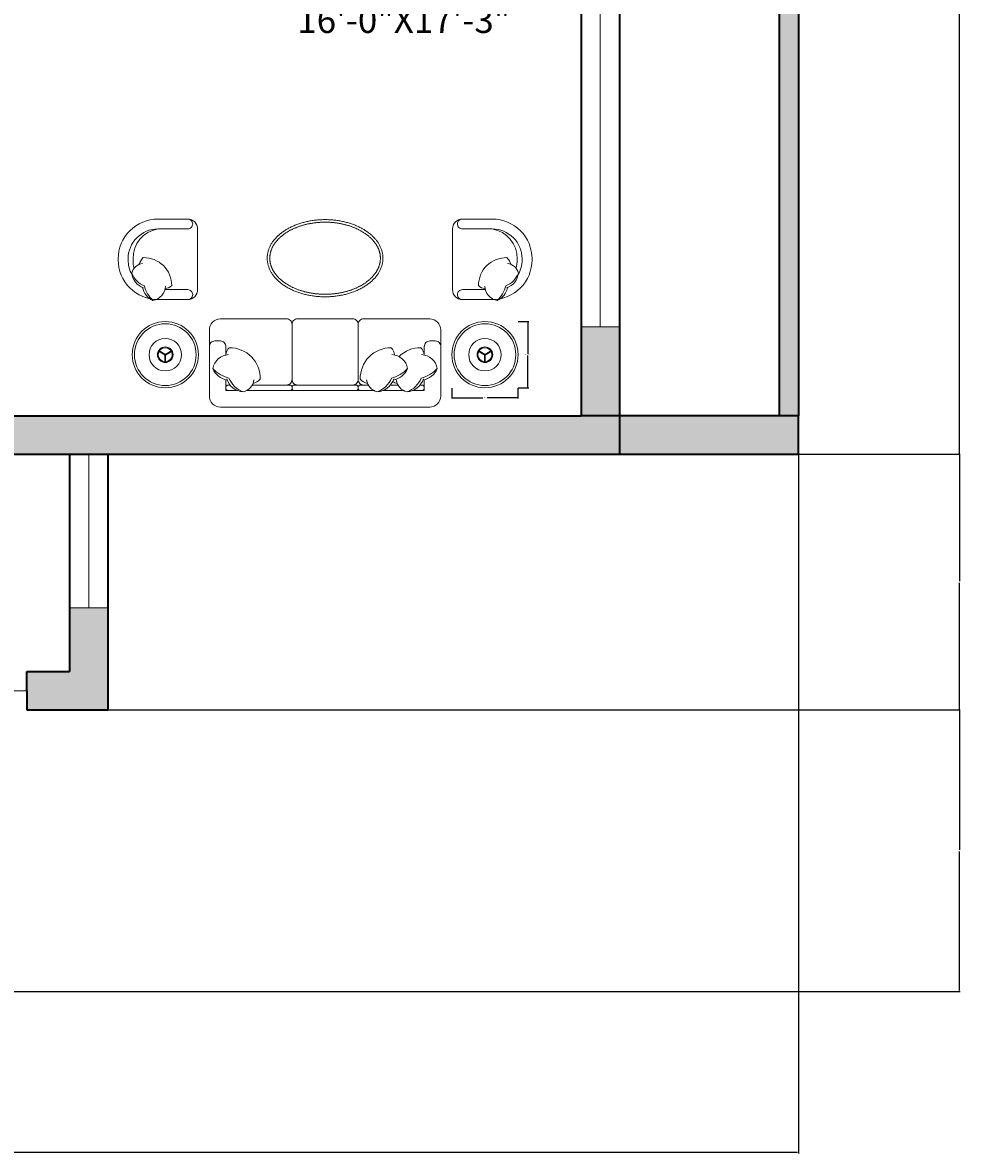
# Model space of a CAD drawing. Units: inches. Extents: x -36 to 442, y -676 to 151.
# Tile 2 of 8: x 222 to 442, y -676 to -411. Entities that reach past the tile are written whole.
import ezdxf

# ---------------------------------------------------------------- set-up
doc = ezdxf.new("R2010")
doc.units = ezdxf.units.IN
doc.header["$MEASUREMENT"] = 0
for name, color, linetype, lineweight in [('A-ANNO-DIMS', 2, 'Continuous', 18), ('A-AREA-IDEN', 7, 'Continuous', 18), ('A-DOOR', 4, 'Continuous', 18), ('A-FURN', 9, 'Continuous', 13), ('A-GLAZ', 4, 'Continuous', 13), ('A-WALL', 7, 'Continuous', 35), ('A-WALL-PATT', 8, 'Continuous', 13)]:
    doc.layers.add(name, color=color, linetype=linetype, lineweight=lineweight)
doc.styles.get("Standard").update_dxf_attribs({"font": 'arial.ttf'})
doc.dimstyles.get("Standard").update_dxf_attribs({"dimtxt": 0.18, "dimasz": 0.18, "dimexe": 0.18, "dimexo": 0.0625, "dimgap": 0.09, "dimtad": 0, "dimtih": 1, "dimtoh": 1, "dimdec": 0, "dimzin": 0, "dimdsep": 46, "dimlunit": 3, "dimtxsty": 'Standard', "dimcen": 0.09, "dimadec": 0, "dimazin": 0, "dimtfac": 1, "dimtdec": 0, "dimtofl": 0, "dimtmove": 0, "dimatfit": 3, "dimfxl": 1, "dimtolj": 1, "dimtzin": 0, "dimarcsym": 0})

# ---------------------------------------------------------------- blocks, each defined once
blk = doc.blocks.new('END-TABLE-ROUND')
at = {"ltscale": 0.03}
for p, q in [((7.72, 7.69), (6.14, 8.6)), ((7.8, 7.83), (6.22, 8.74)), ((7.72, 7.83), (9.3, 8.74)), ((7.8, 7.69), (9.38, 8.6)), ((7.68, 7.76), (7.68, 5.93)), ((7.84, 7.76), (7.84, 5.93))]:
    blk.add_line(p, q, dxfattribs=at)
for radius in [7.76, 3.81, 1.83, 1.64]:
    blk.add_circle((7.76, 7.76), radius, dxfattribs=at)
blk.add_circle((7.76, 7.76), 7.24)
blk = doc.blocks.new('GLAZING-UNIT-36IN')
for p, q in [((0, 36), (0, 0)), ((4.5, 36), (4.5, 0)), ((9, 0), (9, 36))]:
    blk.add_line(p, q)
blk = doc.blocks.new('GLAZING-UNIT-96IN')
for p, q in [((0, 0), (0, 96)), ((4.5, 96), (4.5, 0)), ((9, 96), (9, 0))]:
    blk.add_line(p, q)
blk = doc.blocks.new('*D41')
at = {"layer": 'A-ANNO-DIMS', "color": 0, "lineweight": -2, "transparency": 16777216}
for p, q in [((338.51, -480.93), (340.96, -480.93)), ((340.78, -481.11), (340.78, -488.51)), ((340.78, -496.27), (340.78, -488.87)), ((338.51, -496.45), (340.96, -496.45))]:
    blk.add_line(p, q, dxfattribs=at)
at = {"layer": 'A-ANNO-DIMS', "color": 0, "transparency": 16777216}
for points in [[(340.75, -481.11), (340.81, -481.11), (340.78, -480.93)], [(340.75, -496.27), (340.81, -496.27), (340.78, -496.45)]]:
    blk.add_solid(points, dxfattribs=at)
at = {"layer": 'Defpoints', "color": 0, "transparency": 16777216}
for p in [(338.45, -480.93), (340.78, -480.93), (338.45, -496.45)]:
    blk.add_point(p, dxfattribs=at)
at = {"layer": 'A-ANNO-DIMS', "color": 0, "transparency": 16777216, "insert": (340.78, -488.69), "char_height": 0.18, "attachment_point": 5}
blk.add_mtext('\\A1;TABLE 16 TYP.', dxfattribs=at)
blk = doc.blocks.new('*D42')
at = {"layer": 'A-ANNO-DIMS', "color": 0, "lineweight": -2, "transparency": 16777216}
for p, q in [((322.94, -496.51), (322.94, -498.96)), ((338.45, -496.51), (338.45, -498.96)), ((323.12, -498.78), (330.17, -498.78)), ((338.27, -498.78), (331.21, -498.78))]:
    blk.add_line(p, q, dxfattribs=at)
at = {"layer": 'A-ANNO-DIMS', "color": 0, "transparency": 16777216}
for points in [[(323.12, -498.75), (323.12, -498.81), (322.94, -498.78)], [(338.27, -498.75), (338.27, -498.81), (338.45, -498.78)]]:
    blk.add_solid(points, dxfattribs=at)
at = {"layer": 'Defpoints', "color": 0, "transparency": 16777216}
for p in [(322.94, -496.45), (338.45, -496.45), (338.45, -498.78)]:
    blk.add_point(p, dxfattribs=at)
at = {"layer": 'A-ANNO-DIMS', "color": 0, "transparency": 16777216, "insert": (330.69, -498.78), "char_height": 0.18, "attachment_point": 5}
blk.add_mtext('\\A1;16 TYP.', dxfattribs=at)
blk = doc.blocks.new('*D49')
at = {"layer": 'A-ANNO-DIMS', "color": 0, "lineweight": -2, "transparency": 16777216}
for p, q in [((2.24, -363.56), (2.24, -675.98)), ((404.24, -512.06), (404.24, -675.98)), ((2.42, -675.8), (202.94, -675.8)), ((404.06, -675.8), (203.53, -675.8))]:
    blk.add_line(p, q, dxfattribs=at)
at = {"layer": 'A-ANNO-DIMS', "color": 0, "transparency": 16777216}
for points in [[(2.42, -675.77), (2.42, -675.83), (2.24, -675.8)], [(404.06, -675.77), (404.06, -675.83), (404.24, -675.8)]]:
    blk.add_solid(points, dxfattribs=at)
at = {"layer": 'Defpoints', "color": 0, "transparency": 16777216}
for p in [(2.24, -363.5), (404.24, -512), (404.24, -675.8)]:
    blk.add_point(p, dxfattribs=at)
at = {"layer": 'A-ANNO-DIMS', "color": 0, "transparency": 16777216, "insert": (203.24, -675.8), "char_height": 0.18, "attachment_point": 5}
blk.add_mtext('\\A1;402', dxfattribs=at)
blk = doc.blocks.new('*D59')
at = {"layer": 'A-ANNO-DIMS', "color": 0, "lineweight": -2, "transparency": 16777216}
for p, q in [((404.3, -287), (442.22, -287)), ((442.04, -287.18), (442.04, -399.32)), ((442.04, -511.82), (442.04, -399.68)), ((404.3, -512), (442.22, -512))]:
    blk.add_line(p, q, dxfattribs=at)
at = {"layer": 'A-ANNO-DIMS', "color": 0, "transparency": 16777216}
for points in [[(442.01, -287.18), (442.07, -287.18), (442.04, -287)], [(442.01, -511.82), (442.07, -511.82), (442.04, -512)]]:
    blk.add_solid(points, dxfattribs=at)
at = {"layer": 'Defpoints', "color": 0, "transparency": 16777216}
for p in [(404.24, -287), (404.24, -512), (442.04, -512)]:
    blk.add_point(p, dxfattribs=at)
at = {"layer": 'A-ANNO-DIMS', "color": 0, "transparency": 16777216, "insert": (442.04, -399.5), "char_height": 0.18, "attachment_point": 5}
blk.add_mtext('\\A1;225', dxfattribs=at)
blk = doc.blocks.new('*D60')
at = {"layer": 'A-ANNO-DIMS', "color": 0, "lineweight": -2, "transparency": 16777216}
for p, q in [((404.3, -512), (442.22, -512)), ((442.04, -512.18), (442.04, -541.82)), ((442.04, -571.82), (442.04, -542.18)), ((242.3, -572), (442.22, -572))]:
    blk.add_line(p, q, dxfattribs=at)
at = {"layer": 'A-ANNO-DIMS', "color": 0, "transparency": 16777216}
for points in [[(442.01, -512.18), (442.07, -512.18), (442.04, -512)], [(442.01, -571.82), (442.07, -571.82), (442.04, -572)]]:
    blk.add_solid(points, dxfattribs=at)
at = {"layer": 'Defpoints', "color": 0, "transparency": 16777216}
for p in [(404.24, -512), (442.04, -512), (242.24, -572)]:
    blk.add_point(p, dxfattribs=at)
at = {"layer": 'A-ANNO-DIMS', "color": 0, "transparency": 16777216, "insert": (442.04, -542), "char_height": 0.18, "attachment_point": 5}
blk.add_mtext('\\A1;60', dxfattribs=at)
blk = doc.blocks.new('*D61')
at = {"layer": 'A-ANNO-DIMS', "color": 0, "lineweight": -2, "transparency": 16777216}
for p, q in [((242.3, -572), (442.22, -572)), ((442.04, -572.18), (442.04, -604.82)), ((442.04, -637.82), (442.04, -605.18)), ((72.8, -638), (442.22, -638))]:
    blk.add_line(p, q, dxfattribs=at)
at = {"layer": 'A-ANNO-DIMS', "color": 0, "transparency": 16777216}
for points in [[(442.01, -572.18), (442.07, -572.18), (442.04, -572)], [(442.01, -637.82), (442.07, -637.82), (442.04, -638)]]:
    blk.add_solid(points, dxfattribs=at)
at = {"layer": 'Defpoints', "color": 0, "transparency": 16777216}
for p in [(242.24, -572), (442.04, -572), (72.74, -638)]:
    blk.add_point(p, dxfattribs=at)
at = {"layer": 'A-ANNO-DIMS', "color": 0, "transparency": 16777216, "insert": (442.04, -605), "char_height": 0.18, "attachment_point": 5}
blk.add_mtext('\\A1;66', dxfattribs=at)

msp = doc.modelspace()

# ---------------------------------------------------------------- hatches: boundary and pattern name
at = {"layer": 'A-WALL-PATT'}
h = msp.add_hatch(color=256, dxfattribs=at)
h.dxf.hatch_style = 1
h.paths.add_polyline_path([(288, 113.503), (193.5, 113.503), (97.5, 113.503), (97.5, 104.864), (106.5, 104.864), (106.5, 104.503), (193.5, 104.503), (193.5, 5.503), (193.5, 1.003), (213.735, 1.003), (213.735, -135.497), (218.235, -135.497), (218.235, 1.003), (251, 1.003), (251, 3.253), (251, 5.503), (198, 5.503), (198, 104.503), (279, 104.503), (279, 104.209), (288, 104.209)])
h.paths.add_polyline_path([(378.735, 81.646), (362.235, 81.646), (288, 81.646), (288, 80.209), (279, 80.209), (279, 5.503), (279, 1.003), (353.235, 1.003), (353.235, 0.242), (362.235, 0.242), (362.235, 5.503), (288, 5.503), (288, 77.146), (362.235, 77.146), (374.235, 77.146), (374.235, 5.503), (362.235, 5.503), (362.235, 1.003), (374.235, 1.003), (378.735, 1.003), (378.735, 5.503), (378.735, 77.146)])
h.paths.add_polyline_path([(362.235, -35.758), (353.235, -35.758), (353.235, -196.997), (218.235, -196.997), (213.735, -196.997), (213.735, -205.997), (218.235, -205.997), (378.735, -205.997), (378.735, -205.779), (387.735, -205.779), (387.735, -202.472), (387.735, -196.997), (378.735, -196.997), (362.235, -196.997)])
h.paths.add_polyline_path([(218.235, -175.497), (215.985, -175.497), (213.735, -175.497), (213.735, -196.997), (218.235, -196.997)], flags=17)
h.paths.add_polyline_path([(158.235, -201.497), (98.235, -201.497), (98.235, -205.997), (158.235, -205.997)])
h.paths.add_polyline_path([(173.735, -130.997), (27.735, -130.997), (27.735, -35.267), (18.735, -35.267), (18.735, -138.68), (27.735, -138.68), (27.735, -135.497), (93.735, -135.497), (93.735, -201.497), (98.235, -201.497), (98.235, -135.497), (158.235, -135.497), (158.235, -173.497), (160.739, -173.497), (162.735, -173.497), (162.735, -135.497), (173.735, -135.497), (173.735, -133.017)])
h.paths.add_polyline_path([(98.235, -201.497), (93.735, -201.497), (93.735, -205.997), (98.235, -205.997)])
h.paths.add_polyline_path([(162.735, -201.497), (158.235, -201.497), (158.235, -205.997), (162.735, -205.997)])
h.paths.add_polyline_path([(63.735, -205.997), (63.735, -201.497), (27.735, -201.497), (27.735, -162.68), (18.735, -162.68), (18.735, -210.497), (63.735, -210.497)])
h.paths.add_polyline_path([(65.735, -203.604), (65.735, -201.497), (63.735, -201.497), (63.735, -205.997), (65.735, -205.997)])
h.paths.add_polyline_path([(165.5, 5.503), (106.5, 5.503), (106.5, 80.864), (97.5, 80.864), (97.5, 81.646), (6.735, 81.646), (2.235, 81.646), (2.235, 77.146), (2.235, 5.503), (2.235, 1.003), (6.735, 1.003), (18.735, 1.003), (18.735, 5.503), (6.735, 5.503), (6.735, 77.146), (97.5, 77.146), (97.5, 5.503), (18.735, 5.503), (18.735, 0.733), (27.735, 0.733), (27.735, 1.003), (165.5, 1.003), (165.5, 3.253)])
h.paths.add_polyline_path([(18.735, -201.497), (6.735, -201.497), (2.235, -201.497), (2.235, -210.497), (2.235, -354.497), (2.235, -363.497), (6.735, -363.497), (18.735, -363.497), (18.735, -358.997), (18.735, -354.497), (6.735, -354.497), (6.735, -210.497), (18.735, -210.497)])
h.paths.add_polyline_path([(63.735, -210.497), (54.735, -210.497), (54.735, -240.747), (63.735, -240.747)])
h.paths.add_polyline_path([(63.735, -336.747), (54.735, -336.747), (54.735, -354.497), (18.735, -354.497), (18.735, -358.997), (18.735, -363.497), (104.735, -363.497), (104.735, -361.247), (104.735, -358.997), (63.735, -358.997)])
h.paths.add_polyline_path([(27.735, -448.151), (18.735, -448.151), (18.735, -637.997), (72.735, -637.997), (72.735, -571.997), (183.235, -571.997), (183.235, -562.997), (57.197, -562.997), (51.735, -562.997), (51.735, -567.497), (57.197, -567.497), (63.735, -567.497), (63.735, -571.997), (63.735, -628.997), (27.735, -628.997), (27.735, -475.997), (27.735, -471.497)])
h.paths.add_polyline_path([(27.735, -363.497), (18.735, -363.497), (18.735, -412.151), (27.735, -412.151)])
h.paths.add_polyline_path([(161.235, -358.997), (132.735, -358.997), (132.735, -363.497), (156.735, -363.497), (156.735, -471.497), (51.735, -471.497), (51.735, -475.997), (63.735, -475.997), (63.735, -534.997), (65.985, -534.997), (68.235, -534.997), (68.235, -475.997), (161.235, -475.997)])
h.paths.add_polyline_path([(161.235, -511.997), (173.235, -511.997), (173.235, -502.997), (161.235, -502.997), (161.235, -475.997), (152.235, -475.997), (152.235, -534.997), (156.735, -534.997), (161.235, -534.997)], flags=17)
h.paths.add_polyline_path([(362.235, -502.997), (353.235, -502.997), (213.235, -502.997), (213.235, -507.497), (213.235, -511.997), (362.235, -511.997)])
h.paths.add_polyline_path([(242.235, -548.019), (233.235, -548.019), (233.235, -562.997), (223.235, -562.997), (223.235, -567.497), (223.235, -571.997), (242.235, -571.997)])
h.paths.add_polyline_path([(404.235, -502.997), (399.735, -502.997), (362.235, -502.997), (362.235, -511.997), (399.735, -511.997), (404.235, -511.997)])
h.paths.add_polyline_path([(362.235, -482.123), (353.235, -482.123), (353.235, -502.997), (362.235, -502.997)])
h.paths.add_polyline_path([(404.235, -295.997), (404.235, -286.997), (387.735, -286.997), (387.735, -295.997), (399.735, -295.997), (399.735, -502.997), (404.235, -502.997)])
h.paths.add_polyline_path([(362.235, -355.863), (353.235, -355.863), (353.235, -386.123), (362.235, -386.123)])
h.paths.add_polyline_path([(387.735, -286.997), (378.735, -286.997), (213.735, -286.997), (213.735, -295.997), (353.235, -295.997), (353.235, -295.863), (362.235, -295.863), (362.235, -295.997), (378.735, -295.997), (387.735, -295.997)])
h.paths.add_polyline_path([(387.735, -241.779), (378.735, -241.779), (378.735, -286.997), (387.735, -286.997)])
h.paths.add_polyline_path([(387.735, -175.497), (362.235, -175.497), (362.235, -184.497), (387.735, -184.497)], flags=17)
h.paths.add_polyline_path([(387.735, -184.497), (383.235, -184.497), (383.235, -192.497), (378.735, -192.497), (366.735, -192.497), (366.735, -184.497), (362.235, -184.497), (362.235, -196.997), (378.735, -196.997), (387.735, -196.997)], flags=17)
h.paths.add_polyline_path([(240.604, 40.967), (282.575, 40.967), (282.575, 63.356), (240.604, 63.356)], flags=25)

# ---------------------------------------------------------------- linework, layer by layer
at = {"layer": 'A-DOOR'}
msp.add_line((220.235, -567.497), (223.235, -567.497), dxfattribs=at)
at = {"layer": 'A-FURN', "ltscale": 0.03}
for points in [[(263.302, -466.323), (263.302, -459.212, 0.4142136), (260.97, -456.88), (253.975, -456.88, 0.4142136), (244.649, -466.207), (244.649, -466.323), (244.649, -466.44, 0.4142136), (253.975, -475.766), (260.97, -475.766, 0.4142136), (263.302, -473.435), (263.302, -466.323)], [(323.093, -466.323), (323.093, -459.212, -0.4142136), (325.425, -456.88), (332.42, -456.88, -0.4142136), (341.746, -466.207), (341.746, -466.323), (341.746, -466.44, -0.4142136), (332.42, -475.766), (325.425, -475.766, -0.4142136), (323.093, -473.435), (323.093, -466.323)]]:
    msp.add_lwpolyline(points, format="xyb", dxfattribs=at)
at = {"layer": 'A-FURN'}
for points in [[(253.975, -459.212), (260.97, -459.212, 0.4142136), (262.136, -458.046), (262.136, -458.046, 0.4142136), (260.97, -456.88)], [(332.42, -459.212), (325.425, -459.212, -0.4142136), (324.259, -458.046), (324.259, -458.046, -0.4142136), (325.425, -456.88)], [(253.975, -459.212, 0.4142136), (246.98, -466.207), (246.98, -466.323)], [(253.975, -459.212, 0.3727189), (248.146, -466.207), (248.146, -466.323)], [(332.42, -459.212, -0.3727189), (338.249, -466.207), (338.249, -466.323)], [(332.42, -459.212, -0.4142136), (339.414, -466.207), (339.414, -466.323)], [(247.903, -469.912, -0.1305915), (246.98, -466.44), (246.98, -466.323)], [(248.397, -468.427, -0.0723842), (248.146, -466.44), (248.146, -466.323)], [(255.666, -473.204, 0.1655406), (257.206, -472.483, 0.4259892), (250.528, -465.935, 0.1215233), (249.607, -467.49, -7.1154643)], [(330.729, -473.204, -0.1655406), (329.189, -472.483, -0.4259892), (335.867, -465.935, -0.1215233), (336.788, -467.49, 7.1154643)], [(337.997, -468.427, 0.0723842), (338.249, -466.44), (338.249, -466.323)], [(338.492, -469.912, 0.1305915), (339.414, -466.44), (339.414, -466.323)], [(250.635, -473.02, -0.3066635), (247.856, -469.543, -0.30633), (250.394, -467.272, 0.8728472)], [(335.76, -473.02, 0.3066635), (338.538, -469.543, 0.30633), (336.001, -467.272, -0.8728472)], [(252.798, -475.957, -0.1477299), (250.795, -472.55, -0.2133428), (247.856, -469.543, -0.1786618)], [(333.596, -475.957, 0.1477299), (335.6, -472.55, 0.2133428), (338.538, -469.543, 0.1786618)], [(255.737, -472.616, -0.3567724), (252.798, -475.957, -0.2495421), (250.377, -472.93, 9.6168803)], [(255.61, -473.435), (260.97, -473.435, -0.4142136), (262.136, -474.601), (262.136, -474.601, -0.4142136), (260.97, -475.766)], [(330.785, -473.435), (325.425, -473.435, 0.4142136), (324.259, -474.601), (324.259, -474.601, 0.4142136), (325.425, -475.766)], [(330.658, -472.616, 0.3567724), (333.596, -475.957, 0.2495421), (336.018, -472.93, -9.6168803)], [(284.146, -495.803, 0.4142136), (285.439, -494.51), (285.439, -481.581, 0.4142136)], [(302.248, -495.803, -0.4142136), (300.955, -494.51), (300.955, -481.581, -0.4142136)], [(266.044, -486.753, -0.4142136), (267.337, -485.46), (268.63, -485.46, -0.4142136), (269.923, -486.753), (269.923, -488.756)], [(269.921, -488.756, -0.1655406), (270.721, -487.048, -0.4259892), (277.982, -494.455, -0.1215233), (276.258, -495.476, 7.1154643)], [(309.509, -488.756, 0.1655406), (308.709, -487.048, 0.4259892), (301.447, -494.455, 0.1215233), (303.171, -495.476, -7.1154643)], [(316.474, -488.756, 0.1655406), (315.674, -487.048, 0.2002311), (310.541, -489.129, 0.1215233)], [(316.471, -488.756), (316.471, -486.753, -0.4142136), (317.764, -485.46), (319.057, -485.46, -0.4142136), (320.35, -486.753)], [(270.572, -488.678, 0.3567724), (266.867, -491.937, 0.2495421), (270.224, -494.623, -9.6168803)], [(308.857, -488.678, -0.3567724), (312.562, -491.937, -0.2495421), (309.205, -494.623, 9.6168803)], [(315.822, -488.678, -0.3567724), (319.527, -491.937, -0.2495421), (316.17, -494.623, 9.6168803)], [(266.867, -491.937, 0.1477299), (270.646, -494.159, 0.2133428), (273.981, -497.418, 0.1786618)], [(312.562, -491.937, -0.1477299), (308.783, -494.159, -0.2133428), (305.449, -497.418, -0.1786618)], [(319.527, -491.937, -0.1477299), (315.748, -494.159, -0.2133428), (312.414, -497.418, -0.1786618)], [(270.91, -495.803), (270.441, -495.803, 0.4142136), (269.923, -496.321), (269.923, -496.579, 0.4142136), (270.441, -497.096)], [(270.124, -494.336, 0.3066635), (273.981, -497.418, 0.30633), (276.5, -494.603, -0.8728472)], [(274.795, -497.096), (284.922, -497.096, 0.4142136), (285.439, -496.579), (285.439, -496.321, 0.4142136), (284.922, -495.803), (276.097, -495.803, 0.4142136)], [(286.732, -495.803, -0.4142136), (285.439, -494.51)], [(299.662, -495.803, 0.4142136), (300.955, -494.51)], [(304.635, -497.096), (301.473, -497.096, -0.4142136), (300.955, -496.579), (300.955, -496.321, -0.4142136), (301.473, -495.803), (303.333, -495.803, -0.4142136)], [(309.305, -494.336, -0.3066635), (305.449, -497.418, -0.30633), (302.929, -494.603, 0.8728472)], [(308.519, -495.803), (310.298, -495.803, -0.4142136)], [(309.052, -494.971, 0.0718654), (310.136, -495.476, -7.1154643)], [(316.27, -494.336, -0.3066635), (312.414, -497.418, -0.30633), (309.894, -494.603, 0.8728472)], [(313.751, -497.096), (316.471, -497.096), (316.471, -494.555, -0.4142136)], [(315.485, -495.803), (315.954, -495.803, -0.4142136), (316.471, -496.321), (316.471, -496.579, -0.4142136), (315.954, -497.096)], [(270.441, -497.096), (272.644, -497.096, 0.4142136)], [(311.6, -497.096), (306.786, -497.096, -0.4142136)], [(315.954, -497.096), (313.751, -497.096, -0.4142136)]]:
    msp.add_lwpolyline(points, format="xyb", dxfattribs=at)
at = {"layer": 'A-FURN', "ltscale": 0.03}
msp.add_lwpolyline([(266.044, -482.874, -0.4142136), (268.63, -480.288), (284.146, -480.288, -0.4142136), (285.439, -481.581, -0.4142136), (286.732, -480.288), (299.662, -480.288, -0.4142136), (300.955, -481.581, -0.4142136), (302.248, -480.288), (317.764, -480.288, -0.4142136), (320.35, -482.874), (320.35, -498.389, -0.4142136), (317.764, -500.975), (268.63, -500.975, -0.4142136), (266.044, -498.389)], format="xyb", close=True, dxfattribs=at)
at = {"layer": 'A-FURN'}
for points in [[(269.923, -494.555), (269.923, -497.096), (272.644, -497.096)], [(274.795, -497.096), (304.635, -497.096)], [(306.786, -497.096), (311.6, -497.096)]]:
    msp.add_lwpolyline(points, dxfattribs=at)
msp.add_lwpolyline([(300.438, -497.096), (285.957, -497.096, -0.4142136), (285.439, -496.579), (285.439, -496.321, -0.4142136), (285.957, -495.803), (300.438, -495.803, -0.4142136), (300.955, -496.321), (300.955, -496.579, -0.4142136)], format="xyb", close=True, dxfattribs=at)
at = {"layer": 'A-FURN', "ltscale": 0.03}
msp.add_polyline3d([(279.621, -466.065, 0), (279.623, -466.236, 0), (279.631, -466.407, 0), (279.643, -466.578, 0), (279.66, -466.749, 0), (279.682, -466.92, 0), (279.708, -467.09, 0), (279.74, -467.26, 0), (279.776, -467.43, 0), (279.817, -467.599, 0), (279.863, -467.767, 0), (279.914, -467.935, 0), (279.97, -468.103, 0), (280.03, -468.269, 0), (280.095, -468.435, 0), (280.164, -468.6, 0), (280.239, -468.764, 0), (280.318, -468.927, 0), (280.401, -469.089, 0), (280.489, -469.249, 0), (280.582, -469.409, 0), (280.679, -469.568, 0), (280.781, -469.725, 0), (280.887, -469.881, 0), (280.997, -470.036, 0), (281.112, -470.189, 0), (281.232, -470.341, 0), (281.355, -470.491, 0), (281.483, -470.639, 0), (281.615, -470.786, 0), (281.751, -470.932, 0), (281.891, -471.075, 0), (282.035, -471.217, 0), (282.184, -471.357, 0), (282.336, -471.495, 0), (282.492, -471.631, 0), (282.652, -471.765, 0), (282.816, -471.897, 0), (282.983, -472.027, 0), (283.154, -472.155, 0), (283.329, -472.28, 0), (283.507, -472.404, 0), (283.689, -472.525, 0), (283.874, -472.644, 0), (284.062, -472.76, 0), (284.254, -472.874, 0), (284.449, -472.986, 0), (284.647, -473.095, 0), (284.848, -473.202, 0), (285.052, -473.306, 0), (285.259, -473.407, 0), (285.469, -473.506, 0), (285.681, -473.602, 0), (285.897, -473.696, 0), (286.115, -473.786, 0), (286.335, -473.874, 0), (286.558, -473.959, 0), (286.783, -474.042, 0), (287.011, -474.121, 0), (287.241, -474.198, 0), (287.473, -474.272, 0), (287.707, -474.342, 0), (287.943, -474.41, 0), (288.18, -474.475, 0), (288.42, -474.537, 0), (288.661, -474.595, 0), (288.904, -474.651, 0), (289.149, -474.704, 0), (289.395, -474.753, 0), (289.642, -474.8, 0), (289.891, -474.843, 0), (290.141, -474.883, 0), (290.391, -474.92, 0), (290.643, -474.954, 0), (290.896, -474.985, 0), (291.15, -475.012, 0), (291.404, -475.036, 0), (291.659, -475.057, 0), (291.915, -475.075, 0), (292.171, -475.09, 0), (292.427, -475.101, 0), (292.684, -475.109, 0), (292.94, -475.114, 0), (293.197, -475.116, 0), (293.454, -475.114, 0), (293.711, -475.109, 0), (293.968, -475.101, 0), (294.224, -475.09, 0), (294.48, -475.075, 0), (294.736, -475.057, 0), (294.991, -475.036, 0), (295.245, -475.012, 0), (295.499, -474.985, 0), (295.751, -474.954, 0), (296.003, -474.92, 0), (296.254, -474.883, 0), (296.504, -474.843, 0), (296.753, -474.8, 0), (297, -474.753, 0), (297.246, -474.704, 0), (297.49, -474.651, 0), (297.733, -474.595, 0), (297.975, -474.537, 0), (298.214, -474.475, 0), (298.452, -474.41, 0), (298.688, -474.342, 0), (298.922, -474.272, 0), (299.154, -474.198, 0), (299.384, -474.121, 0), (299.611, -474.042, 0), (299.837, -473.959, 0), (300.06, -473.874, 0), (300.28, -473.786, 0), (300.498, -473.696, 0), (300.713, -473.602, 0), (300.926, -473.506, 0), (301.136, -473.407, 0), (301.343, -473.306, 0), (301.547, -473.202, 0), (301.748, -473.095, 0), (301.946, -472.986, 0), (302.141, -472.874, 0), (302.333, -472.76, 0), (302.521, -472.644, 0), (302.706, -472.525, 0), (302.888, -472.404, 0), (303.066, -472.28, 0), (303.241, -472.155, 0), (303.412, -472.027, 0), (303.579, -471.897, 0), (303.743, -471.765, 0), (303.903, -471.631, 0), (304.059, -471.495, 0), (304.211, -471.357, 0), (304.359, -471.217, 0), (304.504, -471.075, 0), (304.644, -470.932, 0), (304.78, -470.786, 0), (304.912, -470.639, 0), (305.04, -470.491, 0), (305.163, -470.341, 0), (305.282, -470.189, 0), (305.397, -470.036, 0), (305.508, -469.881, 0), (305.614, -469.725, 0), (305.716, -469.568, 0), (305.813, -469.409, 0), (305.906, -469.249, 0), (305.994, -469.089, 0), (306.077, -468.927, 0), (306.156, -468.764, 0), (306.23, -468.6, 0), (306.3, -468.435, 0), (306.365, -468.269, 0), (306.425, -468.103, 0), (306.481, -467.935, 0), (306.531, -467.767, 0), (306.577, -467.599, 0), (306.618, -467.43, 0), (306.655, -467.26, 0), (306.686, -467.09, 0), (306.713, -466.92, 0), (306.735, -466.749, 0), (306.752, -466.578, 0), (306.764, -466.407, 0), (306.771, -466.236, 0), (306.774, -466.065, 0), (306.771, -465.893, 0), (306.764, -465.722, 0), (306.752, -465.551, 0), (306.735, -465.38, 0), (306.713, -465.209, 0), (306.686, -465.039, 0), (306.655, -464.869, 0), (306.618, -464.7, 0), (306.577, -464.53, 0), (306.531, -464.362, 0), (306.481, -464.194, 0), (306.425, -464.027, 0), (306.365, -463.86, 0), (306.3, -463.695, 0), (306.23, -463.53, 0), (306.156, -463.366, 0), (306.077, -463.203, 0), (305.994, -463.041, 0), (305.906, -462.88, 0), (305.813, -462.72, 0), (305.716, -462.561, 0), (305.614, -462.404, 0), (305.508, -462.248, 0), (305.397, -462.094, 0), (305.282, -461.94, 0), (305.163, -461.789, 0), (305.04, -461.638, 0), (304.912, -461.49, 0), (304.78, -461.343, 0), (304.644, -461.198, 0), (304.504, -461.054, 0), (304.359, -460.912, 0), (304.211, -460.772, 0), (304.059, -460.634, 0), (303.903, -460.498, 0), (303.743, -460.364, 0), (303.579, -460.232, 0), (303.412, -460.102, 0), (303.241, -459.974, 0), (303.066, -459.849, 0), (302.888, -459.725, 0), (302.706, -459.604, 0), (302.521, -459.486, 0), (302.333, -459.369, 0), (302.141, -459.255, 0), (301.946, -459.143, 0), (301.748, -459.034, 0), (301.547, -458.928, 0), (301.343, -458.824, 0), (301.136, -458.722, 0), (300.926, -458.623, 0), (300.713, -458.527, 0), (300.498, -458.434, 0), (300.28, -458.343, 0), (300.06, -458.255, 0), (299.837, -458.17, 0), (299.611, -458.087, 0), (299.384, -458.008, 0), (299.154, -457.931, 0), (298.922, -457.858, 0), (298.688, -457.787, 0), (298.452, -457.719, 0), (298.214, -457.654, 0), (297.975, -457.593, 0), (297.733, -457.534, 0), (297.49, -457.478, 0), (297.246, -457.425, 0), (297, -457.376, 0), (296.753, -457.33, 0), (296.504, -457.286, 0), (296.254, -457.246, 0), (296.003, -457.209, 0), (295.751, -457.175, 0), (295.499, -457.145, 0), (295.245, -457.117, 0), (294.991, -457.093, 0), (294.736, -457.072, 0), (294.48, -457.054, 0), (294.224, -457.04, 0), (293.968, -457.028, 0), (293.711, -457.02, 0), (293.454, -457.015, 0), (293.197, -457.014, 0), (292.94, -457.015, 0), (292.684, -457.02, 0), (292.427, -457.028, 0), (292.171, -457.04, 0), (291.915, -457.054, 0), (291.659, -457.072, 0), (291.404, -457.093, 0), (291.15, -457.117, 0), (290.896, -457.145, 0), (290.643, -457.175, 0), (290.391, -457.209, 0), (290.141, -457.246, 0), (289.891, -457.286, 0), (289.642, -457.33, 0), (289.395, -457.376, 0), (289.149, -457.425, 0), (288.904, -457.478, 0), (288.661, -457.534, 0), (288.42, -457.593, 0), (288.18, -457.654, 0), (287.943, -457.719, 0), (287.707, -457.787, 0), (287.473, -457.858, 0), (287.241, -457.931, 0), (287.011, -458.008, 0), (286.783, -458.087, 0), (286.558, -458.17, 0), (286.335, -458.255, 0), (286.115, -458.343, 0), (285.897, -458.434, 0), (285.681, -458.527, 0), (285.469, -458.623, 0), (285.259, -458.722, 0), (285.052, -458.824, 0), (284.848, -458.928, 0), (284.647, -459.034, 0), (284.449, -459.143, 0), (284.254, -459.255, 0), (284.062, -459.369, 0), (283.874, -459.486, 0), (283.689, -459.604, 0), (283.507, -459.725, 0), (283.329, -459.849, 0), (283.154, -459.974, 0), (282.983, -460.102, 0), (282.816, -460.232, 0), (282.652, -460.364, 0), (282.492, -460.498, 0), (282.336, -460.634, 0), (282.184, -460.772, 0), (282.035, -460.912, 0), (281.891, -461.054, 0), (281.751, -461.198, 0), (281.615, -461.343, 0), (281.483, -461.49, 0), (281.355, -461.638, 0), (281.232, -461.789, 0), (281.112, -461.94, 0), (280.997, -462.094, 0), (280.887, -462.248, 0), (280.781, -462.404, 0), (280.679, -462.561, 0), (280.582, -462.72, 0), (280.489, -462.88, 0), (280.401, -463.041, 0), (280.318, -463.203, 0), (280.239, -463.366, 0), (280.164, -463.53, 0), (280.095, -463.695, 0), (280.03, -463.86, 0), (279.97, -464.027, 0), (279.914, -464.194, 0), (279.863, -464.362, 0), (279.817, -464.53, 0), (279.776, -464.7, 0), (279.74, -464.869, 0), (279.708, -465.039, 0), (279.682, -465.209, 0), (279.66, -465.38, 0), (279.643, -465.551, 0), (279.631, -465.722, 0), (279.623, -465.893, 0), (279.621, -466.065, 0)], dxfattribs=at)
at = {"layer": 'A-FURN'}
msp.add_polyline3d([(280.224, -466.065, 0), (280.225, -466.157, 0), (280.227, -466.25, 0), (280.232, -466.344, 0), (280.237, -466.437, 0), (280.244, -466.532, 0), (280.253, -466.626, 0), (280.264, -466.721, 0), (280.276, -466.816, 0), (280.291, -466.912, 0), (280.307, -467.008, 0), (280.324, -467.104, 0), (280.344, -467.201, 0), (280.365, -467.298, 0), (280.388, -467.395, 0), (280.413, -467.492, 0), (280.44, -467.59, 0), (280.469, -467.688, 0), (280.5, -467.786, 0), (280.532, -467.884, 0), (280.567, -467.982, 0), (280.604, -468.081, 0), (280.642, -468.18, 0), (280.683, -468.279, 0), (280.726, -468.378, 0), (280.771, -468.477, 0), (280.818, -468.576, 0), (280.867, -468.675, 0), (280.918, -468.774, 0), (280.971, -468.873, 0), (281.026, -468.972, 0), (281.083, -469.071, 0), (281.143, -469.17, 0), (281.204, -469.268, 0), (281.268, -469.367, 0), (281.333, -469.465, 0), (281.401, -469.562, 0), (281.471, -469.66, 0), (281.542, -469.757, 0), (281.616, -469.854, 0), (281.692, -469.951, 0), (281.77, -470.047, 0), (281.851, -470.142, 0), (281.933, -470.238, 0), (282.018, -470.332, 0), (282.105, -470.426, 0), (282.194, -470.52, 0), (282.285, -470.613, 0), (282.379, -470.706, 0), (282.474, -470.798, 0), (282.572, -470.889, 0), (282.672, -470.98, 0), (282.773, -471.07, 0), (282.877, -471.159, 0), (282.982, -471.247, 0), (283.09, -471.335, 0), (283.199, -471.422, 0), (283.31, -471.508, 0), (283.423, -471.594, 0), (283.538, -471.678, 0), (283.655, -471.762, 0), (283.773, -471.844, 0), (283.893, -471.926, 0), (284.014, -472.007, 0), (284.138, -472.087, 0), (284.262, -472.166, 0), (284.389, -472.243, 0), (284.517, -472.32, 0), (284.646, -472.396, 0), (284.777, -472.47, 0), (284.909, -472.544, 0), (285.043, -472.616, 0), (285.178, -472.687, 0), (285.314, -472.757, 0), (285.452, -472.826, 0), (285.591, -472.893, 0), (285.731, -472.96, 0), (285.872, -473.024, 0), (286.015, -473.088, 0), (286.159, -473.15, 0), (286.303, -473.211, 0), (286.449, -473.27, 0), (286.596, -473.328, 0), (286.744, -473.385, 0), (286.893, -473.44, 0), (287.042, -473.494, 0), (287.192, -473.546, 0), (287.342, -473.597, 0), (287.493, -473.646, 0), (287.643, -473.694, 0), (287.795, -473.74, 0), (287.946, -473.785, 0), (288.098, -473.829, 0), (288.25, -473.871, 0), (288.403, -473.912, 0), (288.556, -473.951, 0), (288.709, -473.989, 0), (288.862, -474.025, 0), (289.016, -474.061, 0), (289.17, -474.094, 0), (289.324, -474.127, 0), (289.479, -474.158, 0), (289.633, -474.188, 0), (289.788, -474.216, 0), (289.944, -474.243, 0), (290.099, -474.269, 0), (290.255, -474.293, 0), (290.411, -474.316, 0), (290.567, -474.338, 0), (290.723, -474.358, 0), (290.879, -474.378, 0), (291.036, -474.395, 0), (291.192, -474.412, 0), (291.349, -474.427, 0), (291.506, -474.441, 0), (291.663, -474.454, 0), (291.82, -474.465, 0), (291.977, -474.475, 0), (292.134, -474.484, 0), (292.292, -474.492, 0), (292.449, -474.498, 0), (292.607, -474.504, 0), (292.764, -474.508, 0), (292.922, -474.51, 0), (293.079, -474.512, 0), (293.237, -474.512, 0), (293.394, -474.511, 0), (293.552, -474.509, 0), (293.709, -474.506, 0), (293.867, -474.501, 0), (294.024, -474.495, 0), (294.182, -474.488, 0), (294.339, -474.48, 0), (294.496, -474.471, 0), (294.653, -474.46, 0), (294.81, -474.448, 0), (294.967, -474.434, 0), (295.124, -474.42, 0), (295.281, -474.404, 0), (295.437, -474.387, 0), (295.594, -474.368, 0), (295.75, -474.348, 0), (295.906, -474.327, 0), (296.062, -474.305, 0), (296.218, -474.281, 0), (296.373, -474.256, 0), (296.529, -474.23, 0), (296.684, -474.202, 0), (296.839, -474.173, 0), (296.993, -474.143, 0), (297.148, -474.111, 0), (297.302, -474.078, 0), (297.456, -474.043, 0), (297.609, -474.007, 0), (297.763, -473.97, 0), (297.916, -473.931, 0), (298.068, -473.891, 0), (298.221, -473.85, 0), (298.373, -473.807, 0), (298.524, -473.763, 0), (298.676, -473.717, 0), (298.827, -473.67, 0), (298.977, -473.621, 0), (299.128, -473.571, 0), (299.277, -473.52, 0), (299.427, -473.467, 0), (299.576, -473.413, 0), (299.724, -473.357, 0), (299.872, -473.3, 0), (300.018, -473.241, 0), (300.164, -473.181, 0), (300.308, -473.119, 0), (300.451, -473.056, 0), (300.593, -472.992, 0), (300.734, -472.927, 0), (300.874, -472.86, 0), (301.012, -472.792, 0), (301.149, -472.722, 0), (301.285, -472.652, 0), (301.419, -472.58, 0), (301.552, -472.507, 0), (301.684, -472.433, 0), (301.814, -472.358, 0), (301.942, -472.282, 0), (302.069, -472.205, 0), (302.195, -472.126, 0), (302.319, -472.047, 0), (302.441, -471.967, 0), (302.562, -471.885, 0), (302.681, -471.803, 0), (302.799, -471.72, 0), (302.914, -471.636, 0), (303.028, -471.551, 0), (303.14, -471.465, 0), (303.25, -471.379, 0), (303.359, -471.291, 0), (303.465, -471.203, 0), (303.57, -471.114, 0), (303.672, -471.025, 0), (303.773, -470.934, 0), (303.872, -470.843, 0), (303.968, -470.752, 0), (304.063, -470.66, 0), (304.155, -470.567, 0), (304.246, -470.473, 0), (304.334, -470.379, 0), (304.419, -470.285, 0), (304.503, -470.19, 0), (304.584, -470.095, 0), (304.664, -469.999, 0), (304.741, -469.902, 0), (304.816, -469.806, 0), (304.889, -469.709, 0), (304.959, -469.611, 0), (305.028, -469.514, 0), (305.095, -469.416, 0), (305.159, -469.317, 0), (305.222, -469.219, 0), (305.282, -469.12, 0), (305.34, -469.022, 0), (305.396, -468.923, 0), (305.451, -468.824, 0), (305.503, -468.725, 0), (305.553, -468.626, 0), (305.601, -468.526, 0), (305.647, -468.427, 0), (305.69, -468.328, 0), (305.732, -468.229, 0), (305.772, -468.13, 0), (305.81, -468.032, 0), (305.845, -467.933, 0), (305.879, -467.835, 0), (305.911, -467.737, 0), (305.94, -467.639, 0), (305.968, -467.541, 0), (305.994, -467.443, 0), (306.018, -467.346, 0), (306.041, -467.249, 0), (306.061, -467.152, 0), (306.08, -467.056, 0), (306.096, -466.96, 0), (306.111, -466.864, 0), (306.125, -466.769, 0), (306.136, -466.674, 0), (306.146, -466.579, 0), (306.154, -466.484, 0), (306.161, -466.39, 0), (306.165, -466.297, 0), (306.169, -466.204, 0), (306.17, -466.111, 0), (306.17, -466.018, 0), (306.169, -465.926, 0), (306.165, -465.832, 0), (306.161, -465.739, 0), (306.154, -465.645, 0), (306.146, -465.55, 0), (306.136, -465.456, 0), (306.125, -465.361, 0), (306.111, -465.265, 0), (306.096, -465.169, 0), (306.08, -465.073, 0), (306.061, -464.977, 0), (306.041, -464.88, 0), (306.018, -464.783, 0), (305.994, -464.686, 0), (305.968, -464.588, 0), (305.94, -464.491, 0), (305.911, -464.393, 0), (305.879, -464.295, 0), (305.845, -464.196, 0), (305.81, -464.098, 0), (305.772, -463.999, 0), (305.732, -463.9, 0), (305.69, -463.801, 0), (305.647, -463.702, 0), (305.601, -463.603, 0), (305.553, -463.504, 0), (305.503, -463.405, 0), (305.451, -463.306, 0), (305.396, -463.207, 0), (305.34, -463.108, 0), (305.282, -463.009, 0), (305.222, -462.91, 0), (305.159, -462.812, 0), (305.095, -462.714, 0), (305.028, -462.616, 0), (304.959, -462.518, 0), (304.889, -462.421, 0), (304.816, -462.324, 0), (304.741, -462.227, 0), (304.664, -462.131, 0), (304.584, -462.035, 0), (304.503, -461.939, 0), (304.419, -461.844, 0), (304.334, -461.75, 0), (304.246, -461.656, 0), (304.155, -461.563, 0), (304.063, -461.47, 0), (303.968, -461.377, 0), (303.872, -461.286, 0), (303.773, -461.195, 0), (303.672, -461.105, 0), (303.57, -461.015, 0), (303.465, -460.926, 0), (303.359, -460.838, 0), (303.25, -460.751, 0), (303.14, -460.664, 0), (303.028, -460.578, 0), (302.914, -460.493, 0), (302.799, -460.409, 0), (302.681, -460.326, 0), (302.562, -460.244, 0), (302.441, -460.163, 0), (302.319, -460.082, 0), (302.195, -460.003, 0), (302.069, -459.925, 0), (301.942, -459.847, 0), (301.814, -459.771, 0), (301.684, -459.696, 0), (301.552, -459.622, 0), (301.419, -459.549, 0), (301.285, -459.477, 0), (301.149, -459.407, 0), (301.012, -459.338, 0), (300.874, -459.269, 0), (300.734, -459.203, 0), (300.593, -459.137, 0), (300.451, -459.073, 0), (300.308, -459.01, 0), (300.164, -458.949, 0), (300.018, -458.888, 0), (299.872, -458.83, 0), (299.724, -458.772, 0), (299.576, -458.717, 0), (299.427, -458.662, 0), (299.277, -458.609, 0), (299.128, -458.558, 0), (298.977, -458.508, 0), (298.827, -458.459, 0), (298.676, -458.412, 0), (298.524, -458.367, 0), (298.373, -458.322, 0), (298.221, -458.279, 0), (298.068, -458.238, 0), (297.916, -458.198, 0), (297.763, -458.159, 0), (297.609, -458.122, 0), (297.456, -458.086, 0), (297.302, -458.052, 0), (297.148, -458.018, 0), (296.993, -457.987, 0), (296.839, -457.956, 0), (296.684, -457.927, 0), (296.529, -457.899, 0), (296.373, -457.873, 0), (296.218, -457.848, 0), (296.062, -457.824, 0), (295.906, -457.802, 0), (295.75, -457.781, 0), (295.594, -457.761, 0), (295.437, -457.743, 0), (295.281, -457.725, 0), (295.124, -457.71, 0), (294.967, -457.695, 0), (294.81, -457.682, 0), (294.653, -457.67, 0), (294.496, -457.659, 0), (294.339, -457.649, 0), (294.182, -457.641, 0), (294.024, -457.634, 0), (293.867, -457.628, 0), (293.709, -457.623, 0), (293.552, -457.62, 0), (293.394, -457.618, 0), (293.237, -457.617, 0), (293.079, -457.617, 0), (292.922, -457.619, 0), (292.764, -457.622, 0), (292.607, -457.626, 0), (292.449, -457.631, 0), (292.292, -457.637, 0), (292.134, -457.645, 0), (291.977, -457.654, 0), (291.82, -457.664, 0), (291.663, -457.675, 0), (291.506, -457.688, 0), (291.349, -457.702, 0), (291.192, -457.717, 0), (291.036, -457.734, 0), (290.879, -457.752, 0), (290.723, -457.771, 0), (290.567, -457.791, 0), (290.411, -457.813, 0), (290.255, -457.836, 0), (290.099, -457.86, 0), (289.944, -457.886, 0), (289.788, -457.913, 0), (289.633, -457.942, 0), (289.479, -457.971, 0), (289.324, -458.002, 0), (289.17, -458.035, 0), (289.016, -458.069, 0), (288.862, -458.104, 0), (288.709, -458.14, 0), (288.556, -458.178, 0), (288.403, -458.218, 0), (288.25, -458.258, 0), (288.098, -458.301, 0), (287.946, -458.344, 0), (287.795, -458.389, 0), (287.643, -458.436, 0), (287.493, -458.483, 0), (287.342, -458.533, 0), (287.192, -458.583, 0), (287.042, -458.636, 0), (286.893, -458.689, 0), (286.744, -458.744, 0), (286.596, -458.801, 0), (286.449, -458.859, 0), (286.303, -458.918, 0), (286.159, -458.979, 0), (286.015, -459.041, 0), (285.872, -459.105, 0), (285.731, -459.17, 0), (285.591, -459.236, 0), (285.452, -459.303, 0), (285.314, -459.372, 0), (285.178, -459.442, 0), (285.043, -459.513, 0), (284.909, -459.585, 0), (284.777, -459.659, 0), (284.646, -459.733, 0), (284.517, -459.809, 0), (284.389, -459.886, 0), (284.262, -459.964, 0), (284.138, -460.043, 0), (284.014, -460.122, 0), (283.893, -460.203, 0), (283.773, -460.285, 0), (283.655, -460.368, 0), (283.538, -460.451, 0), (283.423, -460.536, 0), (283.31, -460.621, 0), (283.199, -460.707, 0), (283.09, -460.794, 0), (282.982, -460.882, 0), (282.877, -460.97, 0), (282.773, -461.06, 0), (282.672, -461.15, 0), (282.572, -461.24, 0), (282.474, -461.332, 0), (282.379, -461.424, 0), (282.285, -461.516, 0), (282.194, -461.609, 0), (282.105, -461.703, 0), (282.018, -461.797, 0), (281.933, -461.892, 0), (281.851, -461.987, 0), (281.77, -462.083, 0), (281.692, -462.179, 0), (281.616, -462.275, 0), (281.542, -462.372, 0), (281.471, -462.469, 0), (281.401, -462.567, 0), (281.333, -462.665, 0), (281.268, -462.763, 0), (281.204, -462.861, 0), (281.143, -462.96, 0), (281.083, -463.058, 0), (281.026, -463.157, 0), (280.971, -463.256, 0), (280.918, -463.355, 0), (280.867, -463.454, 0), (280.818, -463.553, 0), (280.771, -463.652, 0), (280.726, -463.752, 0), (280.683, -463.851, 0), (280.642, -463.949, 0), (280.604, -464.048, 0), (280.567, -464.147, 0), (280.532, -464.245, 0), (280.5, -464.344, 0), (280.469, -464.442, 0), (280.44, -464.54, 0), (280.413, -464.637, 0), (280.388, -464.735, 0), (280.365, -464.832, 0), (280.344, -464.929, 0), (280.324, -465.025, 0), (280.307, -465.121, 0), (280.291, -465.217, 0), (280.276, -465.313, 0), (280.264, -465.408, 0), (280.253, -465.503, 0), (280.244, -465.598, 0), (280.237, -465.692, 0), (280.232, -465.786, 0), (280.227, -465.879, 0), (280.225, -465.972, 0), (280.224, -466.065, 0)], dxfattribs=at)
at = {"layer": 'A-GLAZ'}
for p, q in [((362.235, -482.123), (353.235, -482.123)), ((242.235, -512.019), (233.235, -512.019)), ((233.235, -548.019), (242.235, -548.019))]:
    msp.add_line(p, q, dxfattribs=at)
at = {"layer": 'A-WALL'}
for p, q in [((353.235, -295.997), (353.235, -502.997)), ((362.235, -295.997), (362.235, -511.997)), ((399.735, -295.997), (399.735, -502.997)), ((404.235, -295.997), (404.235, -502.997)), ((213.235, -502.997), (353.235, -502.997)), ((399.735, -502.997), (353.235, -502.997)), ((404.235, -502.997), (399.735, -502.997)), ((404.235, -511.997), (404.235, -502.997)), ((213.235, -511.997), (362.235, -511.997)), ((233.235, -511.997), (233.235, -562.997)), ((242.235, -511.997), (242.235, -571.997)), ((362.235, -511.997), (399.735, -511.997)), ((399.735, -511.997), (404.235, -511.997)), ((223.235, -562.997), (233.235, -562.997)), ((223.235, -567.497), (223.235, -562.997)), ((223.235, -567.497), (223.235, -571.997)), ((223.235, -571.997), (242.235, -571.997))]:
    msp.add_line(p, q, dxfattribs=at)

# ---------------------------------------------------------------- block references
at = {"layer": 'A-FURN'}
for p in [(247.943, -496.45), (322.937, -496.45)]:
    msp.add_blockref('END-TABLE-ROUND', p, dxfattribs=at)
at = {"layer": 'A-GLAZ'}
for name, p in [('GLAZING-UNIT-96IN', (353.235, -482.123)), ('GLAZING-UNIT-36IN', (233.235, -548.019))]:
    msp.add_blockref(name, p, dxfattribs=at)

# ---------------------------------------------------------------- texts
at = {"layer": 'A-AREA-IDEN', "insert": (286.694, -397.246), "char_height": 6, "attachment_point": 1}
msp.add_mtext('LIVING\\P16\'-0"X17\'-3"', dxfattribs=at)

# ---------------------------------------------------------------- dimensions: what is measured, and where the dimension line sits
at = {"layer": 'A-ANNO-DIMS'}
for base, p1, p2, picture, middle in [((442.035, -511.997), (404.235, -286.997), (404.235, -511.997), '*D59', (442.035, -399.497)), ((442.035, -511.997), (242.235, -571.997), (404.235, -511.997), '*D60', (442.035, -541.997)), ((442.035, -571.997), (72.735, -637.997), (242.235, -571.997), '*D61', (442.035, -604.997))]:
    dim = msp.add_linear_dim(base=base, p1=p1, p2=p2, angle=90, dimstyle='Standard', override={"dimdec": 0, "dimlfac": 1, "dimrnd": 0, "dimzin": 0, "dimdsep": 46, "dimlunit": 2}, dxfattribs=at)
    dim.commit()
    dim.dimension.update_dxf_attribs({"geometry": picture, "text_midpoint": middle})
dim = msp.add_linear_dim(base=(404.235, -675.797), p1=(2.235, -363.497), p2=(404.235, -511.997), dimstyle='Standard', override={"dimdec": 0, "dimlfac": 1, "dimrnd": 0, "dimzin": 0, "dimdsep": 46, "dimlunit": 2}, dxfattribs=at)
dim.commit()
dim.dimension.update_dxf_attribs({"geometry": '*D49', "text_midpoint": (203.235, -675.797)})
dim = msp.add_linear_dim(base=(340.78, -480.934), p1=(338.452, -496.45), p2=(338.452, -480.934), angle=90, text='TABLE <> TYP.', dimstyle='Standard', override={"dimdec": 0, "dimlfac": 1, "dimrnd": 0, "dimzin": 0, "dimdsep": 46, "dimlunit": 2}, dxfattribs=at)
dim.commit()
dim.dimension.update_dxf_attribs({"geometry": '*D41', "text_midpoint": (340.78, -488.692)})
dim = msp.add_linear_dim(base=(338.452, -498.777), p1=(322.936, -496.45), p2=(338.452, -496.45), text='<> TYP.', dimstyle='Standard', override={"dimdec": 0, "dimlfac": 1, "dimrnd": 0, "dimzin": 0, "dimdsep": 46, "dimlunit": 2}, dxfattribs=at)
dim.commit()
dim.dimension.update_dxf_attribs({"geometry": '*D42', "text_midpoint": (330.694, -498.777)})

doc.saveas('drawing.dxf')
